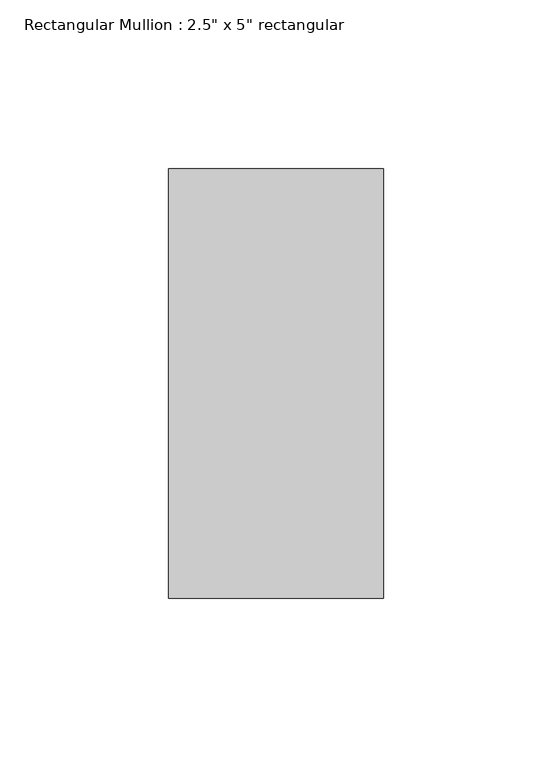
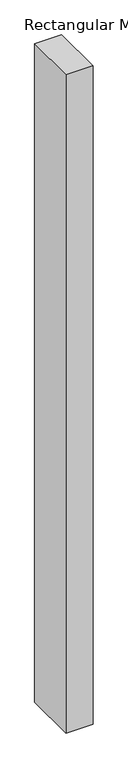
"""IFC4 building model written with IfcOpenShell, lengths in millimetres: member geometry."""

from ifc_helpers import new_model, si_unit, frame, origin, place, context, project, spatial, polyline, outline, extrude, source, transform, mapped, element, save


def member_ee21581d(model_context):
    return source(origin(), model_context, "Body", "SweptSolid", [
        extrude(outline(polyline([(31.75, 63.5), (31.75, -63.5), (-31.75, -63.5), (-31.75, 63.5), (31.75, 63.5)])), frame((0.0, 0.0, -1630.931829), z_axis=(0.0, 0.0, 1.0), x_axis=(1.0, 0.0, 0.0)), (0.0, 0.0, 1.0), 1630.931829),
    ])


if __name__ == "__main__":
    model = new_model("IFC4")
    model_context = context("Model", 3, world=origin())
    ifc_project = project(units=[si_unit("LENGTHUNIT", "METRE", prefix="MILLI")], contexts=[model_context])
    site = spatial("IfcSite", under=ifc_project)
    building = spatial("IfcBuilding", under=site)
    placement = place(None, origin())
    member_shape = member_ee21581d(model_context)
    element("IfcMember", 1, ObjectType="Rectangular Mullion : 2.5\" x 5\" rectangular", at=placement, inside=building, context=model_context, shape_type="MappedRepresentation", body=[
        mapped(member_shape, transform((0.0, 0.0, 0.0), x_axis=(1.0, 0.0, 0.0), y_axis=(0.0, 1.0, 0.0), z_axis=(0.0, 0.0, 1.0))),
    ])
    save(model, "model.ifc")

# Revit data of these elements
# Type "Rectangular Mullion : 2.5\" x 5\" rectangular"
#   built-in parameter 1007304 = 0.416667 (stored number, unit not read)
#   built-in parameter 1007301 = 0.104167 (stored number, unit not read)
#   built-in parameter 1007300 = 0.104167 (stored number, unit not read)
# Element 1 (IfcMember, "Rectangular Mullion : 2.5\" x 5\" rectangular")
#   Materials on its faces: "Aluminum"
# Materials
#   "Aluminum": class "Metal", colour RGB 247 247 247, transparency 0, Description = "Aluminum 6061", Cost = 0
